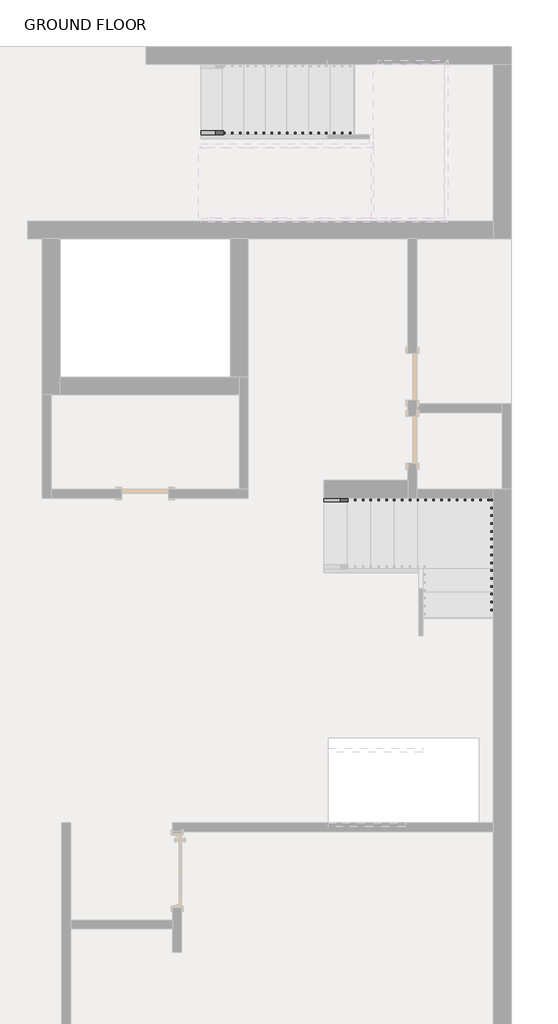
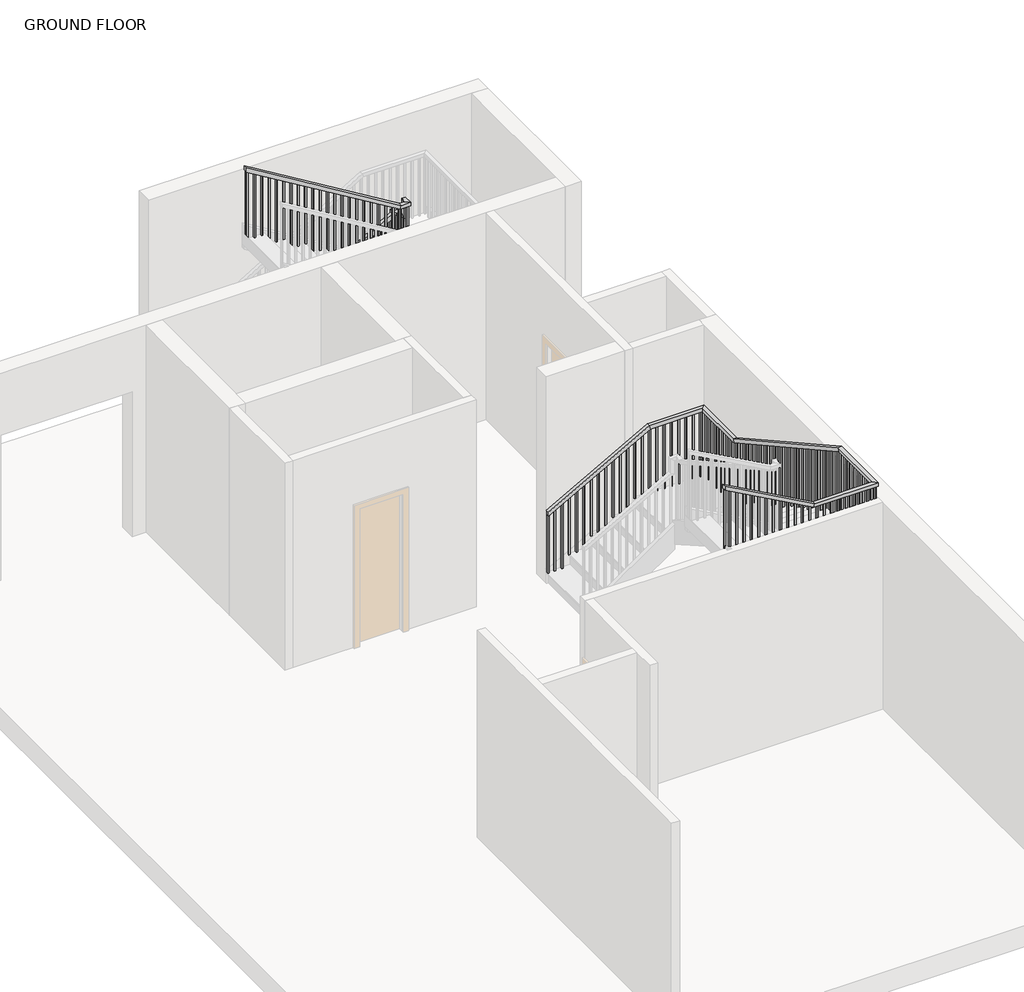
# One storey, part 2 of 3: 2 railings.
"""IFC4 building model written with IfcOpenShell, lengths in millimetres."""

from ifc_helpers import new_model, si_unit, frame, origin, place, context, project, spatial, polyline, outline, extrude, faceted_brep, element, save

model = new_model("IFC4")

# Units and contexts
model_context = context("Model", 3, world=origin())
ifc_project = project(units=[si_unit("LENGTHUNIT", "METRE", prefix="MILLI")], contexts=[model_context])

# Site, building, storey
site = spatial("IfcSite", under=ifc_project)
building = spatial("IfcBuilding", under=site)
storey = spatial("IfcBuildingStorey", under=building, Name="GROUND FLOOR", Elevation=304.8)

# Railings
placement = place(None, origin())
element("IfcRailing", 1, ObjectType="Handrail - Rectangular", at=placement, inside=storey, context=model_context, shape_type="SolidModel", body=[
    faceted_brep([(-12941.4571222, 6804.8964313, 1388.5333333), (-12941.4571222, 6804.8964313, 1329.1318731), (-12941.4571222, 6754.0964313, 1329.1318731), (-12941.4571222, 6754.0964313, 1388.5333333), (-10782.4571222, 6804.8964313, 2697.0181818), (-10731.6571222, 6804.8964313, 2668.4046004), (-10731.6571222, 6754.0964313, 2668.4046004), (-10782.4571222, 6754.0964313, 2697.0181818), (-10782.4571222, 6804.8964313, 2743.2), (-10731.6571222, 6804.8964313, 2692.4), (-10731.6571222, 6754.0964313, 2692.4), (-10782.4571222, 6754.0964313, 2743.2), (-10655.4571222, 6804.8964313, 2743.2), (-10655.4571222, 6804.8964313, 2692.4), (-10706.2571222, 6754.0964313, 2692.4), (-10706.2571222, 6754.0964313, 2743.2), (-10655.4571222, 6677.8964313, 2743.2), (-10655.4571222, 6677.8964313, 2692.4), (-10706.2571222, 6677.8964313, 2692.4), (-10706.2571222, 6677.8964313, 2743.2), (-10655.4571222, 6663.5776214, 2743.2), (-10655.4571222, 6612.7776214, 2692.4), (-10706.2571222, 6612.7776214, 2692.4), (-10706.2571222, 6663.5776214, 2743.2), (-10655.4571222, 6663.5776214, 2958.7151515), (-10655.4571222, 6612.7776214, 2907.9151515), (-10706.2571222, 6612.7776214, 2907.9151515), (-10706.2571222, 6663.5776214, 2958.7151515), (-10655.4571222, 6536.5776214, 2958.7151515), (-10655.4571222, 6536.5776214, 2907.9151515), (-10706.2571222, 6587.3776214, 2907.9151515), (-10706.2571222, 6587.3776214, 2958.7151515), (-10782.4571222, 6536.5776214, 2958.7151515), (-10796.6495316, 6536.5776214, 2907.9151515), (-10796.6495316, 6587.3776214, 2907.9151515), (-10782.4571222, 6587.3776214, 2958.7151515), (-12941.4571222, 6536.5776214, 4267.2), (-12941.4571222, 6587.3776214, 4267.2), (-12941.4571222, 6587.3776214, 4207.7985397), (-12941.4571222, 6536.5776214, 4207.7985397)], [[[0, 1, 2, 3]], [[1, 0, 4, 5]], [[2, 1, 5, 6]], [[3, 2, 6, 7]], [[0, 3, 7, 4]], [[5, 4, 8, 9]], [[6, 5, 9, 10]], [[7, 6, 10, 11]], [[4, 7, 11, 8]], [[9, 8, 12, 13]], [[10, 9, 13, 14]], [[11, 10, 14, 15]], [[8, 11, 15, 12]], [[13, 12, 16, 17]], [[14, 13, 17, 18]], [[15, 14, 18, 19]], [[12, 15, 19, 16]], [[17, 16, 20, 21]], [[18, 17, 21, 22]], [[19, 18, 22, 23]], [[16, 19, 23, 20]], [[21, 20, 24, 25]], [[22, 21, 25, 26]], [[23, 22, 26, 27]], [[20, 23, 27, 24]], [[25, 24, 28, 29]], [[26, 25, 29, 30]], [[27, 26, 30, 31]], [[24, 27, 31, 28]], [[29, 28, 32, 33]], [[30, 29, 33, 34]], [[31, 30, 34, 35]], [[28, 31, 35, 32]], [[36, 37, 38, 39]], [[33, 32, 36, 39]], [[34, 33, 39, 38]], [[35, 34, 38, 37]], [[32, 35, 37, 36]]]),
    extrude(outline(polyline([(4186.6318731, -12906.5321222), (4198.1773276, -12925.5821222), (3183.4666667, -12925.5821222), (3183.4666667, -12906.5321222), (4186.6318731, -12906.5321222)])), frame((0.0, 6552.4526214, 0.0), z_axis=(0.0, 1.0, 0.0), x_axis=(0.0, 0.0, 1.0)), (0.0, 0.0, 1.0), 19.05),
    extrude(outline(polyline([(4125.0561155, -12804.9321222), (4136.60157, -12823.9821222), (3183.4666667, -12823.9821222), (3183.4666667, -12804.9321222), (4125.0561155, -12804.9321222)])), frame((0.0, 6552.4526214, 0.0), z_axis=(0.0, 1.0, 0.0), x_axis=(0.0, 0.0, 1.0)), (0.0, 0.0, 1.0), 19.05),
    extrude(outline(polyline([(4063.4803579, -12703.3321222), (4075.0258125, -12722.3821222), (3183.4666667, -12722.3821222), (3183.4666667, -12703.3321222), (4063.4803579, -12703.3321222)])), frame((0.0, 6552.4526214, 0.0), z_axis=(0.0, 1.0, 0.0), x_axis=(0.0, 0.0, 1.0)), (0.0, 0.0, 1.0), 19.05),
    extrude(outline(polyline([(4001.9046004, -12601.7321222), (4013.4500549, -12620.7821222), (3014.1333333, -12620.7821222), (3014.1333333, -12601.7321222), (4001.9046004, -12601.7321222)])), frame((0.0, 6552.4526214, 0.0), z_axis=(0.0, 1.0, 0.0), x_axis=(0.0, 0.0, 1.0)), (0.0, 0.0, 1.0), 19.05),
    extrude(outline(polyline([(3940.3288428, -12500.1321222), (3951.8742973, -12519.1821222), (3014.1333333, -12519.1821222), (3014.1333333, -12500.1321222), (3940.3288428, -12500.1321222)])), frame((0.0, 6552.4526214, 0.0), z_axis=(0.0, 1.0, 0.0), x_axis=(0.0, 0.0, 1.0)), (0.0, 0.0, 1.0), 19.05),
    extrude(outline(polyline([(3878.7530852, -12398.5321222), (3890.2985397, -12417.5821222), (3014.1333333, -12417.5821222), (3014.1333333, -12398.5321222), (3878.7530852, -12398.5321222)])), frame((0.0, 6552.4526214, 0.0), z_axis=(0.0, 1.0, 0.0), x_axis=(0.0, 0.0, 1.0)), (0.0, 0.0, 1.0), 19.05),
    extrude(outline(polyline([(3817.1773276, -12296.9321222), (3828.7227822, -12315.9821222), (2844.8, -12315.9821222), (2844.8, -12296.9321222), (3817.1773276, -12296.9321222)])), frame((0.0, 6552.4526214, 0.0), z_axis=(0.0, 1.0, 0.0), x_axis=(0.0, 0.0, 1.0)), (0.0, 0.0, 1.0), 19.05),
    extrude(outline(polyline([(3755.60157, -12195.3321222), (3767.1470246, -12214.3821222), (2844.8, -12214.3821222), (2844.8, -12195.3321222), (3755.60157, -12195.3321222)])), frame((0.0, 6552.4526214, 0.0), z_axis=(0.0, 1.0, 0.0), x_axis=(0.0, 0.0, 1.0)), (0.0, 0.0, 1.0), 19.05),
    extrude(outline(polyline([(3694.0258125, -12093.7321222), (3705.571267, -12112.7821222), (2844.8, -12112.7821222), (2844.8, -12093.7321222), (3694.0258125, -12093.7321222)])), frame((0.0, 6552.4526214, 0.0), z_axis=(0.0, 1.0, 0.0), x_axis=(0.0, 0.0, 1.0)), (0.0, 0.0, 1.0), 19.05),
    extrude(outline(polyline([(3632.4500549, -11992.1321222), (3643.9955094, -12011.1821222), (2675.4666667, -12011.1821222), (2675.4666667, -11992.1321222), (3632.4500549, -11992.1321222)])), frame((0.0, 6552.4526214, 0.0), z_axis=(0.0, 1.0, 0.0), x_axis=(0.0, 0.0, 1.0)), (0.0, 0.0, 1.0), 19.05),
    extrude(outline(polyline([(3570.8742973, -11890.5321222), (3582.4197519, -11909.5821222), (2675.4666667, -11909.5821222), (2675.4666667, -11890.5321222), (3570.8742973, -11890.5321222)])), frame((0.0, 6552.4526214, 0.0), z_axis=(0.0, 1.0, 0.0), x_axis=(0.0, 0.0, 1.0)), (0.0, 0.0, 1.0), 19.05),
    extrude(outline(polyline([(3509.2985397, -11788.9321222), (3520.8439943, -11807.9821222), (2506.1333333, -11807.9821222), (2506.1333333, -11788.9321222), (3509.2985397, -11788.9321222)])), frame((0.0, 6552.4526214, 0.0), z_axis=(0.0, 1.0, 0.0), x_axis=(0.0, 0.0, 1.0)), (0.0, 0.0, 1.0), 19.05),
    extrude(outline(polyline([(3447.7227822, -11687.3321222), (3459.2682367, -11706.3821222), (2506.1333333, -11706.3821222), (2506.1333333, -11687.3321222), (3447.7227822, -11687.3321222)])), frame((0.0, 6552.4526214, 0.0), z_axis=(0.0, 1.0, 0.0), x_axis=(0.0, 0.0, 1.0)), (0.0, 0.0, 1.0), 19.05),
    extrude(outline(polyline([(3386.1470246, -11585.7321222), (3397.6924791, -11604.7821222), (2506.1333333, -11604.7821222), (2506.1333333, -11585.7321222), (3386.1470246, -11585.7321222)])), frame((0.0, 6552.4526214, 0.0), z_axis=(0.0, 1.0, 0.0), x_axis=(0.0, 0.0, 1.0)), (0.0, 0.0, 1.0), 19.05),
    extrude(outline(polyline([(3324.571267, -11484.1321222), (3336.1167216, -11503.1821222), (2336.8, -11503.1821222), (2336.8, -11484.1321222), (3324.571267, -11484.1321222)])), frame((0.0, 6552.4526214, 0.0), z_axis=(0.0, 1.0, 0.0), x_axis=(0.0, 0.0, 1.0)), (0.0, 0.0, 1.0), 19.05),
    extrude(outline(polyline([(3262.9955094, -11382.5321222), (3274.540964, -11401.5821222), (2336.8, -11401.5821222), (2336.8, -11382.5321222), (3262.9955094, -11382.5321222)])), frame((0.0, 6552.4526214, 0.0), z_axis=(0.0, 1.0, 0.0), x_axis=(0.0, 0.0, 1.0)), (0.0, 0.0, 1.0), 19.05),
    extrude(outline(polyline([(3201.4197519, -11280.9321222), (3212.9652064, -11299.9821222), (2336.8, -11299.9821222), (2336.8, -11280.9321222), (3201.4197519, -11280.9321222)])), frame((0.0, 6552.4526214, 0.0), z_axis=(0.0, 1.0, 0.0), x_axis=(0.0, 0.0, 1.0)), (0.0, 0.0, 1.0), 19.05),
    extrude(outline(polyline([(3139.8439943, -11179.3321222), (3151.3894488, -11198.3821222), (2167.4666667, -11198.3821222), (2167.4666667, -11179.3321222), (3139.8439943, -11179.3321222)])), frame((0.0, 6552.4526214, 0.0), z_axis=(0.0, 1.0, 0.0), x_axis=(0.0, 0.0, 1.0)), (0.0, 0.0, 1.0), 19.05),
    extrude(outline(polyline([(3078.2682367, -11077.7321222), (3089.8136913, -11096.7821222), (2167.4666667, -11096.7821222), (2167.4666667, -11077.7321222), (3078.2682367, -11077.7321222)])), frame((0.0, 6552.4526214, 0.0), z_axis=(0.0, 1.0, 0.0), x_axis=(0.0, 0.0, 1.0)), (0.0, 0.0, 1.0), 19.05),
    extrude(outline(polyline([(3016.6924791, -10976.1321222), (3028.2379337, -10995.1821222), (2167.4666667, -10995.1821222), (2167.4666667, -10976.1321222), (3016.6924791, -10976.1321222)])), frame((0.0, 6552.4526214, 0.0), z_axis=(0.0, 1.0, 0.0), x_axis=(0.0, 0.0, 1.0)), (0.0, 0.0, 1.0), 19.05),
    extrude(outline(polyline([(2955.1167216, -10874.5321222), (2966.6621761, -10893.5821222), (1998.1333333, -10893.5821222), (1998.1333333, -10874.5321222), (2955.1167216, -10874.5321222)])), frame((0.0, 6552.4526214, 0.0), z_axis=(0.0, 1.0, 0.0), x_axis=(0.0, 0.0, 1.0)), (0.0, 0.0, 1.0), 19.05),
    extrude(outline(polyline([(2893.540964, -10772.9321222), (2905.0864185, -10791.9821222), (1998.1333333, -10791.9821222), (1998.1333333, -10772.9321222), (2893.540964, -10772.9321222)])), frame((0.0, 6552.4526214, 0.0), z_axis=(0.0, 1.0, 0.0), x_axis=(0.0, 0.0, 1.0)), (0.0, 0.0, 1.0), 19.05),
    extrude(outline(polyline([(-10690.3821222, 6585.8214313), (-10671.3321222, 6585.8214313), (-10671.3321222, 6566.7714313), (-10690.3821222, 6566.7714313), (-10690.3821222, 6585.8214313)])), frame((0.0, 0.0, 1828.8), z_axis=(0.0, 0.0, 1.0), x_axis=(1.0, 0.0, 0.0)), (0.0, 0.0, 1.0), 1079.1151515),
    extrude(outline(polyline([(-10690.3821222, 6687.4214313), (-10671.3321222, 6687.4214313), (-10671.3321222, 6668.3714313), (-10690.3821222, 6668.3714313), (-10690.3821222, 6687.4214313)])), frame((0.0, 0.0, 1828.8), z_axis=(0.0, 0.0, 1.0), x_axis=(1.0, 0.0, 0.0)), (0.0, 0.0, 1.0), 863.6),
    extrude(outline(polyline([(-10715.7821222, 6769.9714313), (-10715.7821222, 6789.0214313), (-10696.7321222, 6789.0214313), (-10696.7321222, 6769.9714313), (-10715.7821222, 6769.9714313)])), frame((0.0, 0.0, 1828.8), z_axis=(0.0, 0.0, 1.0), x_axis=(1.0, 0.0, 0.0)), (0.0, 0.0, 1.0), 863.6),
    extrude(outline(polyline([(2627.9955094, -10798.3321222), (2616.4500549, -10817.3821222), (1659.4666667, -10817.3821222), (1659.4666667, -10798.3321222), (2627.9955094, -10798.3321222)])), frame((0.0, 6769.9714313, 0.0), z_axis=(0.0, 1.0, 0.0), x_axis=(0.0, 0.0, 1.0)), (0.0, 0.0, 1.0), 19.05),
    extrude(outline(polyline([(2566.4197519, -10899.9321222), (2554.8742973, -10918.9821222), (1659.4666667, -10918.9821222), (1659.4666667, -10899.9321222), (2566.4197519, -10899.9321222)])), frame((0.0, 6769.9714313, 0.0), z_axis=(0.0, 1.0, 0.0), x_axis=(0.0, 0.0, 1.0)), (0.0, 0.0, 1.0), 19.05),
    extrude(outline(polyline([(2504.8439943, -11001.5321222), (2493.2985397, -11020.5821222), (1490.1333333, -11020.5821222), (1490.1333333, -11001.5321222), (2504.8439943, -11001.5321222)])), frame((0.0, 6769.9714313, 0.0), z_axis=(0.0, 1.0, 0.0), x_axis=(0.0, 0.0, 1.0)), (0.0, 0.0, 1.0), 19.05),
    extrude(outline(polyline([(2443.2682367, -11103.1321222), (2431.7227822, -11122.1821222), (1490.1333333, -11122.1821222), (1490.1333333, -11103.1321222), (2443.2682367, -11103.1321222)])), frame((0.0, 6769.9714313, 0.0), z_axis=(0.0, 1.0, 0.0), x_axis=(0.0, 0.0, 1.0)), (0.0, 0.0, 1.0), 19.05),
    extrude(outline(polyline([(2381.6924791, -11204.7321222), (2370.1470246, -11223.7821222), (1490.1333333, -11223.7821222), (1490.1333333, -11204.7321222), (2381.6924791, -11204.7321222)])), frame((0.0, 6769.9714313, 0.0), z_axis=(0.0, 1.0, 0.0), x_axis=(0.0, 0.0, 1.0)), (0.0, 0.0, 1.0), 19.05),
    extrude(outline(polyline([(2320.1167216, -11306.3321222), (2308.571267, -11325.3821222), (1320.8, -11325.3821222), (1320.8, -11306.3321222), (2320.1167216, -11306.3321222)])), frame((0.0, 6769.9714313, 0.0), z_axis=(0.0, 1.0, 0.0), x_axis=(0.0, 0.0, 1.0)), (0.0, 0.0, 1.0), 19.05),
    extrude(outline(polyline([(2258.540964, -11407.9321222), (2246.9955094, -11426.9821222), (1320.8, -11426.9821222), (1320.8, -11407.9321222), (2258.540964, -11407.9321222)])), frame((0.0, 6769.9714313, 0.0), z_axis=(0.0, 1.0, 0.0), x_axis=(0.0, 0.0, 1.0)), (0.0, 0.0, 1.0), 19.05),
    extrude(outline(polyline([(2196.9652064, -11509.5321222), (2185.4197519, -11528.5821222), (1320.8, -11528.5821222), (1320.8, -11509.5321222), (2196.9652064, -11509.5321222)])), frame((0.0, 6769.9714313, 0.0), z_axis=(0.0, 1.0, 0.0), x_axis=(0.0, 0.0, 1.0)), (0.0, 0.0, 1.0), 19.05),
    extrude(outline(polyline([(2135.3894488, -11611.1321222), (2123.8439943, -11630.1821222), (1151.4666667, -11630.1821222), (1151.4666667, -11611.1321222), (2135.3894488, -11611.1321222)])), frame((0.0, 6769.9714313, 0.0), z_axis=(0.0, 1.0, 0.0), x_axis=(0.0, 0.0, 1.0)), (0.0, 0.0, 1.0), 19.05),
    extrude(outline(polyline([(2073.8136913, -11712.7321222), (2062.2682367, -11731.7821222), (1151.4666667, -11731.7821222), (1151.4666667, -11712.7321222), (2073.8136913, -11712.7321222)])), frame((0.0, 6769.9714313, 0.0), z_axis=(0.0, 1.0, 0.0), x_axis=(0.0, 0.0, 1.0)), (0.0, 0.0, 1.0), 19.05),
    extrude(outline(polyline([(2012.2379337, -11814.3321222), (2000.6924791, -11833.3821222), (1151.4666667, -11833.3821222), (1151.4666667, -11814.3321222), (2012.2379337, -11814.3321222)])), frame((0.0, 6769.9714313, 0.0), z_axis=(0.0, 1.0, 0.0), x_axis=(0.0, 0.0, 1.0)), (0.0, 0.0, 1.0), 19.05),
    extrude(outline(polyline([(1950.6621761, -11915.9321222), (1939.1167216, -11934.9821222), (982.1333333, -11934.9821222), (982.1333333, -11915.9321222), (1950.6621761, -11915.9321222)])), frame((0.0, 6769.9714313, 0.0), z_axis=(0.0, 1.0, 0.0), x_axis=(0.0, 0.0, 1.0)), (0.0, 0.0, 1.0), 19.05),
    extrude(outline(polyline([(1889.0864185, -12017.5321222), (1877.540964, -12036.5821222), (982.1333333, -12036.5821222), (982.1333333, -12017.5321222), (1889.0864185, -12017.5321222)])), frame((0.0, 6769.9714313, 0.0), z_axis=(0.0, 1.0, 0.0), x_axis=(0.0, 0.0, 1.0)), (0.0, 0.0, 1.0), 19.05),
    extrude(outline(polyline([(1827.510661, -12119.1321222), (1815.9652064, -12138.1821222), (812.8, -12138.1821222), (812.8, -12119.1321222), (1827.510661, -12119.1321222)])), frame((0.0, 6769.9714313, 0.0), z_axis=(0.0, 1.0, 0.0), x_axis=(0.0, 0.0, 1.0)), (0.0, 0.0, 1.0), 19.05),
    extrude(outline(polyline([(1765.9349034, -12220.7321222), (1754.3894488, -12239.7821222), (812.8, -12239.7821222), (812.8, -12220.7321222), (1765.9349034, -12220.7321222)])), frame((0.0, 6769.9714313, 0.0), z_axis=(0.0, 1.0, 0.0), x_axis=(0.0, 0.0, 1.0)), (0.0, 0.0, 1.0), 19.05),
    extrude(outline(polyline([(1704.3591458, -12322.3321222), (1692.8136913, -12341.3821222), (812.8, -12341.3821222), (812.8, -12322.3321222), (1704.3591458, -12322.3321222)])), frame((0.0, 6769.9714313, 0.0), z_axis=(0.0, 1.0, 0.0), x_axis=(0.0, 0.0, 1.0)), (0.0, 0.0, 1.0), 19.05),
    extrude(outline(polyline([(1642.7833882, -12423.9321222), (1631.2379337, -12442.9821222), (643.4666667, -12442.9821222), (643.4666667, -12423.9321222), (1642.7833882, -12423.9321222)])), frame((0.0, 6769.9714313, 0.0), z_axis=(0.0, 1.0, 0.0), x_axis=(0.0, 0.0, 1.0)), (0.0, 0.0, 1.0), 19.05),
    extrude(outline(polyline([(1581.2076307, -12525.5321222), (1569.6621761, -12544.5821222), (643.4666667, -12544.5821222), (643.4666667, -12525.5321222), (1581.2076307, -12525.5321222)])), frame((0.0, 6769.9714313, 0.0), z_axis=(0.0, 1.0, 0.0), x_axis=(0.0, 0.0, 1.0)), (0.0, 0.0, 1.0), 19.05),
    extrude(outline(polyline([(1519.6318731, -12627.1321222), (1508.0864185, -12646.1821222), (643.4666667, -12646.1821222), (643.4666667, -12627.1321222), (1519.6318731, -12627.1321222)])), frame((0.0, 6769.9714313, 0.0), z_axis=(0.0, 1.0, 0.0), x_axis=(0.0, 0.0, 1.0)), (0.0, 0.0, 1.0), 19.05),
    extrude(outline(polyline([(1458.0561155, -12728.7321222), (1446.510661, -12747.7821222), (474.1333333, -12747.7821222), (474.1333333, -12728.7321222), (1458.0561155, -12728.7321222)])), frame((0.0, 6769.9714313, 0.0), z_axis=(0.0, 1.0, 0.0), x_axis=(0.0, 0.0, 1.0)), (0.0, 0.0, 1.0), 19.05),
    extrude(outline(polyline([(1396.4803579, -12830.3321222), (1384.9349034, -12849.3821222), (474.1333333, -12849.3821222), (474.1333333, -12830.3321222), (1396.4803579, -12830.3321222)])), frame((0.0, 6769.9714313, 0.0), z_axis=(0.0, 1.0, 0.0), x_axis=(0.0, 0.0, 1.0)), (0.0, 0.0, 1.0), 19.05),
    extrude(outline(polyline([(-10690.3821222, 6571.5026214), (-10671.3321222, 6571.5026214), (-10671.3321222, 6552.4526214), (-10690.3821222, 6552.4526214), (-10690.3821222, 6571.5026214)])), frame((0.0, 0.0, 1828.8), z_axis=(0.0, 0.0, 1.0), x_axis=(1.0, 0.0, 0.0)), (0.0, 0.0, 1.0), 1079.1151515),
    extrude(outline(polyline([(-10690.3821222, 6769.9714313), (-10690.3821222, 6789.0214313), (-10671.3321222, 6789.0214313), (-10671.3321222, 6769.9714313), (-10690.3821222, 6769.9714313)])), frame((0.0, 0.0, 1828.8), z_axis=(0.0, 0.0, 1.0), x_axis=(1.0, 0.0, 0.0)), (0.0, 0.0, 1.0), 863.6),
    extrude(outline(polyline([(4196.2530852, -12922.4071222), (4207.7985397, -12941.4571222), (3183.4666667, -12941.4571222), (3183.4666667, -12922.4071222), (4196.2530852, -12922.4071222)])), frame((0.0, 6552.4526214, 0.0), z_axis=(0.0, 1.0, 0.0), x_axis=(0.0, 0.0, 1.0)), (0.0, 0.0, 1.0), 19.05),
    extrude(outline(polyline([(1340.6773276, -12922.4071222), (1329.1318731, -12941.4571222), (474.1333333, -12941.4571222), (474.1333333, -12922.4071222), (1340.6773276, -12922.4071222)])), frame((0.0, 6769.9714313, 0.0), z_axis=(0.0, 1.0, 0.0), x_axis=(0.0, 0.0, 1.0)), (0.0, 0.0, 1.0), 19.05),
])
element("IfcRailing", 2, ObjectType="Handrail - Rectangular", at=placement, inside=storey, context=model_context, shape_type="SolidModel", body=[
    faceted_brep([(-11350.6229553, 2055.0964313, 1388.5333333), (-11350.6229553, 2055.0964313, 1330.420221), (-11350.6229553, 2004.2964313, 1330.420221), (-11350.6229553, 2004.2964313, 1388.5333333), (-9947.2729553, 2055.0964313, 2168.1722222), (-9934.109353, 2055.0964313, 2117.3722222), (-9934.109353, 2004.2964313, 2117.3722222), (-9947.2729553, 2004.2964313, 2168.1722222), (-9153.5229553, 2055.0964313, 2168.1722222), (-9153.5229553, 2055.0964313, 2117.3722222), (-9204.3229553, 2004.2964313, 2117.3722222), (-9204.3229553, 2004.2964313, 2168.1722222), (-9153.5229553, 1261.3464313, 2168.1722222), (-9153.5229553, 1248.1828291, 2117.3722222), (-9204.3229553, 1248.1828291, 2117.3722222), (-9204.3229553, 1261.3464313, 2168.1722222), (-9153.5229553, -1265.9535687, 3572.2277778), (-9153.5229553, -1279.1171709, 3521.4277778), (-9204.3229553, -1279.1171709, 3521.4277778), (-9204.3229553, -1265.9535687, 3572.2277778), (-9153.5229553, -2148.6035687, 3572.2277778), (-9153.5229553, -2148.6035687, 3521.4277778), (-9204.3229553, -2097.8035687, 3521.4277778), (-9204.3229553, -2097.8035687, 3572.2277778), (-10036.1729553, -2148.6035687, 3572.2277778), (-10049.3365575, -2148.6035687, 3521.4277778), (-10049.3365575, -2097.8035687, 3521.4277778), (-10036.1729553, -2097.8035687, 3572.2277778), (-11287.1229553, -2148.6035687, 4267.2), (-11287.1229553, -2097.8035687, 4267.2), (-11287.1229553, -2097.8035687, 4209.0868876), (-11287.1229553, -2148.6035687, 4209.0868876)], [[[0, 1, 2, 3]], [[1, 0, 4, 5]], [[2, 1, 5, 6]], [[3, 2, 6, 7]], [[0, 3, 7, 4]], [[5, 4, 8, 9]], [[6, 5, 9, 10]], [[7, 6, 10, 11]], [[4, 7, 11, 8]], [[9, 8, 12, 13]], [[10, 9, 13, 14]], [[11, 10, 14, 15]], [[8, 11, 15, 12]], [[13, 12, 16, 17]], [[14, 13, 17, 18]], [[15, 14, 18, 19]], [[12, 15, 19, 16]], [[17, 16, 20, 21]], [[18, 17, 21, 22]], [[19, 18, 22, 23]], [[16, 19, 23, 20]], [[21, 20, 24, 25]], [[22, 21, 25, 26]], [[23, 22, 26, 27]], [[20, 23, 27, 24]], [[28, 29, 30, 31]], [[25, 24, 28, 31]], [[26, 25, 31, 30]], [[27, 26, 30, 29]], [[24, 27, 29, 28]]]),
    extrude(outline(polyline([(4172.045221, -11220.4479553), (3183.4666667, -11220.4479553), (3183.4666667, -11201.3979553), (4161.4618876, -11201.3979553), (4172.045221, -11220.4479553)])), frame((0.0, -2132.7285687, 0.0), z_axis=(0.0, 1.0, 0.0), x_axis=(0.0, 0.0, 1.0)), (0.0, 0.0, 1.0), 19.05),
    extrude(outline(polyline([(4115.6007765, -11118.8479553), (3183.4666667, -11118.8479553), (3183.4666667, -11099.7979553), (4105.0174432, -11099.7979553), (4115.6007765, -11118.8479553)])), frame((0.0, -2132.7285687, 0.0), z_axis=(0.0, 1.0, 0.0), x_axis=(0.0, 0.0, 1.0)), (0.0, 0.0, 1.0), 19.05),
    extrude(outline(polyline([(4059.1563321, -11017.2479553), (3183.4666667, -11017.2479553), (3183.4666667, -10998.1979553), (4048.5729988, -10998.1979553), (4059.1563321, -11017.2479553)])), frame((0.0, -2132.7285687, 0.0), z_axis=(0.0, 1.0, 0.0), x_axis=(0.0, 0.0, 1.0)), (0.0, 0.0, 1.0), 19.05),
    extrude(outline(polyline([(4002.7118876, -10915.6479553), (3014.1333333, -10915.6479553), (3014.1333333, -10896.5979553), (3992.1285543, -10896.5979553), (4002.7118876, -10915.6479553)])), frame((0.0, -2132.7285687, 0.0), z_axis=(0.0, 1.0, 0.0), x_axis=(0.0, 0.0, 1.0)), (0.0, 0.0, 1.0), 19.05),
    extrude(outline(polyline([(3946.2674432, -10814.0479553), (3014.1333333, -10814.0479553), (3014.1333333, -10794.9979553), (3935.6841099, -10794.9979553), (3946.2674432, -10814.0479553)])), frame((0.0, -2132.7285687, 0.0), z_axis=(0.0, 1.0, 0.0), x_axis=(0.0, 0.0, 1.0)), (0.0, 0.0, 1.0), 19.05),
    extrude(outline(polyline([(3889.8229988, -10712.4479553), (3014.1333333, -10712.4479553), (3014.1333333, -10693.3979553), (3879.2396654, -10693.3979553), (3889.8229988, -10712.4479553)])), frame((0.0, -2132.7285687, 0.0), z_axis=(0.0, 1.0, 0.0), x_axis=(0.0, 0.0, 1.0)), (0.0, 0.0, 1.0), 19.05),
    extrude(outline(polyline([(3833.3785543, -10610.8479553), (2844.8, -10610.8479553), (2844.8, -10591.7979553), (3822.795221, -10591.7979553), (3833.3785543, -10610.8479553)])), frame((0.0, -2132.7285687, 0.0), z_axis=(0.0, 1.0, 0.0), x_axis=(0.0, 0.0, 1.0)), (0.0, 0.0, 1.0), 19.05),
    extrude(outline(polyline([(3776.9341099, -10509.2479553), (2844.8, -10509.2479553), (2844.8, -10490.1979553), (3766.3507765, -10490.1979553), (3776.9341099, -10509.2479553)])), frame((0.0, -2132.7285687, 0.0), z_axis=(0.0, 1.0, 0.0), x_axis=(0.0, 0.0, 1.0)), (0.0, 0.0, 1.0), 19.05),
    extrude(outline(polyline([(3720.4896654, -10407.6479553), (2844.8, -10407.6479553), (2844.8, -10388.5979553), (3709.9063321, -10388.5979553), (3720.4896654, -10407.6479553)])), frame((0.0, -2132.7285687, 0.0), z_axis=(0.0, 1.0, 0.0), x_axis=(0.0, 0.0, 1.0)), (0.0, 0.0, 1.0), 19.05),
    extrude(outline(polyline([(3664.045221, -10306.0479553), (2675.4666667, -10306.0479553), (2675.4666667, -10286.9979553), (3653.4618876, -10286.9979553), (3664.045221, -10306.0479553)])), frame((0.0, -2132.7285687, 0.0), z_axis=(0.0, 1.0, 0.0), x_axis=(0.0, 0.0, 1.0)), (0.0, 0.0, 1.0), 19.05),
    extrude(outline(polyline([(3607.6007765, -10204.4479553), (2675.4666667, -10204.4479553), (2675.4666667, -10185.3979553), (3597.0174432, -10185.3979553), (3607.6007765, -10204.4479553)])), frame((0.0, -2132.7285687, 0.0), z_axis=(0.0, 1.0, 0.0), x_axis=(0.0, 0.0, 1.0)), (0.0, 0.0, 1.0), 19.05),
    extrude(outline(polyline([(3551.1563321, -10102.8479553), (2675.4666667, -10102.8479553), (2675.4666667, -10083.7979553), (3540.5729988, -10083.7979553), (3551.1563321, -10102.8479553)])), frame((0.0, -2132.7285687, 0.0), z_axis=(0.0, 1.0, 0.0), x_axis=(0.0, 0.0, 1.0)), (0.0, 0.0, 1.0), 19.05),
    extrude(outline(polyline([(-9982.1979553, -2132.7285687), (-10001.2479553, -2132.7285687), (-10001.2479553, -2113.6785687), (-9982.1979553, -2113.6785687), (-9982.1979553, -2132.7285687)])), frame((0.0, 0.0, 2506.1333333), z_axis=(0.0, 0.0, 1.0), x_axis=(1.0, 0.0, 0.0)), (0.0, 0.0, 1.0), 1015.2944444),
    extrude(outline(polyline([(-9880.5979553, -2132.7285687), (-9899.6479553, -2132.7285687), (-9899.6479553, -2113.6785687), (-9880.5979553, -2113.6785687), (-9880.5979553, -2132.7285687)])), frame((0.0, 0.0, 2506.1333333), z_axis=(0.0, 0.0, 1.0), x_axis=(1.0, 0.0, 0.0)), (0.0, 0.0, 1.0), 1015.2944444),
    extrude(outline(polyline([(-9778.9979553, -2132.7285687), (-9798.0479553, -2132.7285687), (-9798.0479553, -2113.6785687), (-9778.9979553, -2113.6785687), (-9778.9979553, -2132.7285687)])), frame((0.0, 0.0, 2506.1333333), z_axis=(0.0, 0.0, 1.0), x_axis=(1.0, 0.0, 0.0)), (0.0, 0.0, 1.0), 1015.2944444),
    extrude(outline(polyline([(-9677.3979553, -2132.7285687), (-9696.4479553, -2132.7285687), (-9696.4479553, -2113.6785687), (-9677.3979553, -2113.6785687), (-9677.3979553, -2132.7285687)])), frame((0.0, 0.0, 2506.1333333), z_axis=(0.0, 0.0, 1.0), x_axis=(1.0, 0.0, 0.0)), (0.0, 0.0, 1.0), 1015.2944444),
    extrude(outline(polyline([(-9575.7979553, -2132.7285687), (-9594.8479553, -2132.7285687), (-9594.8479553, -2113.6785687), (-9575.7979553, -2113.6785687), (-9575.7979553, -2132.7285687)])), frame((0.0, 0.0, 2506.1333333), z_axis=(0.0, 0.0, 1.0), x_axis=(1.0, 0.0, 0.0)), (0.0, 0.0, 1.0), 1015.2944444),
    extrude(outline(polyline([(-9474.1979553, -2132.7285687), (-9493.2479553, -2132.7285687), (-9493.2479553, -2113.6785687), (-9474.1979553, -2113.6785687), (-9474.1979553, -2132.7285687)])), frame((0.0, 0.0, 2506.1333333), z_axis=(0.0, 0.0, 1.0), x_axis=(1.0, 0.0, 0.0)), (0.0, 0.0, 1.0), 1015.2944444),
    extrude(outline(polyline([(-9372.5979553, -2132.7285687), (-9391.6479553, -2132.7285687), (-9391.6479553, -2113.6785687), (-9372.5979553, -2113.6785687), (-9372.5979553, -2132.7285687)])), frame((0.0, 0.0, 2506.1333333), z_axis=(0.0, 0.0, 1.0), x_axis=(1.0, 0.0, 0.0)), (0.0, 0.0, 1.0), 1015.2944444),
    extrude(outline(polyline([(-9270.9979553, -2132.7285687), (-9290.0479553, -2132.7285687), (-9290.0479553, -2113.6785687), (-9270.9979553, -2113.6785687), (-9270.9979553, -2132.7285687)])), frame((0.0, 0.0, 2506.1333333), z_axis=(0.0, 0.0, 1.0), x_axis=(1.0, 0.0, 0.0)), (0.0, 0.0, 1.0), 1015.2944444),
    extrude(outline(polyline([(-9169.3979553, -2024.7785687), (-9169.3979553, -2043.8285687), (-9188.4479553, -2043.8285687), (-9188.4479553, -2024.7785687), (-9169.3979553, -2024.7785687)])), frame((0.0, 0.0, 2506.1333333), z_axis=(0.0, 0.0, 1.0), x_axis=(1.0, 0.0, 0.0)), (0.0, 0.0, 1.0), 1015.2944444),
    extrude(outline(polyline([(-9169.3979553, -1923.1785687), (-9169.3979553, -1942.2285687), (-9188.4479553, -1942.2285687), (-9188.4479553, -1923.1785687), (-9169.3979553, -1923.1785687)])), frame((0.0, 0.0, 2506.1333333), z_axis=(0.0, 0.0, 1.0), x_axis=(1.0, 0.0, 0.0)), (0.0, 0.0, 1.0), 1015.2944444),
    extrude(outline(polyline([(-9169.3979553, -1821.5785687), (-9169.3979553, -1840.6285687), (-9188.4479553, -1840.6285687), (-9188.4479553, -1821.5785687), (-9169.3979553, -1821.5785687)])), frame((0.0, 0.0, 2506.1333333), z_axis=(0.0, 0.0, 1.0), x_axis=(1.0, 0.0, 0.0)), (0.0, 0.0, 1.0), 1015.2944444),
    extrude(outline(polyline([(-9169.3979553, -1719.9785687), (-9169.3979553, -1739.0285687), (-9188.4479553, -1739.0285687), (-9188.4479553, -1719.9785687), (-9169.3979553, -1719.9785687)])), frame((0.0, 0.0, 2506.1333333), z_axis=(0.0, 0.0, 1.0), x_axis=(1.0, 0.0, 0.0)), (0.0, 0.0, 1.0), 1015.2944444),
    extrude(outline(polyline([(-9169.3979553, -1618.3785687), (-9169.3979553, -1637.4285687), (-9188.4479553, -1637.4285687), (-9188.4479553, -1618.3785687), (-9169.3979553, -1618.3785687)])), frame((0.0, 0.0, 2506.1333333), z_axis=(0.0, 0.0, 1.0), x_axis=(1.0, 0.0, 0.0)), (0.0, 0.0, 1.0), 1015.2944444),
    extrude(outline(polyline([(-9169.3979553, -1516.7785687), (-9169.3979553, -1535.8285687), (-9188.4479553, -1535.8285687), (-9188.4479553, -1516.7785687), (-9169.3979553, -1516.7785687)])), frame((0.0, 0.0, 2506.1333333), z_axis=(0.0, 0.0, 1.0), x_axis=(1.0, 0.0, 0.0)), (0.0, 0.0, 1.0), 1015.2944444),
    extrude(outline(polyline([(-9169.3979553, -1415.1785687), (-9169.3979553, -1434.2285687), (-9188.4479553, -1434.2285687), (-9188.4479553, -1415.1785687), (-9169.3979553, -1415.1785687)])), frame((0.0, 0.0, 2506.1333333), z_axis=(0.0, 0.0, 1.0), x_axis=(1.0, 0.0, 0.0)), (0.0, 0.0, 1.0), 1015.2944444),
    extrude(outline(polyline([(-9169.3979553, -1313.5785687), (-9169.3979553, -1332.6285687), (-9188.4479553, -1332.6285687), (-9188.4479553, -1313.5785687), (-9169.3979553, -1313.5785687)])), frame((0.0, 0.0, 2506.1333333), z_axis=(0.0, 0.0, 1.0), x_axis=(1.0, 0.0, 0.0)), (0.0, 0.0, 1.0), 1015.2944444),
    extrude(outline(polyline([(-1211.9785687, 3484.1285543), (-1211.9785687, 2506.1333333), (-1231.0285687, 2506.1333333), (-1231.0285687, 3494.7118876), (-1211.9785687, 3484.1285543)])), frame((-9188.4479553, 0.0, 0.0), z_axis=(1.0, 0.0, 0.0), x_axis=(0.0, 1.0, 0.0)), (0.0, 0.0, 1.0), 19.05),
    extrude(outline(polyline([(-1110.3785687, 3427.6841099), (-1110.3785687, 2506.1333333), (-1129.4285687, 2506.1333333), (-1129.4285687, 3438.2674432), (-1110.3785687, 3427.6841099)])), frame((-9188.4479553, 0.0, 0.0), z_axis=(1.0, 0.0, 0.0), x_axis=(0.0, 1.0, 0.0)), (0.0, 0.0, 1.0), 19.05),
    extrude(outline(polyline([(-1008.7785687, 3371.2396654), (-1008.7785687, 2506.1333333), (-1027.8285687, 2506.1333333), (-1027.8285687, 3381.8229988), (-1008.7785687, 3371.2396654)])), frame((-9188.4479553, 0.0, 0.0), z_axis=(1.0, 0.0, 0.0), x_axis=(0.0, 1.0, 0.0)), (0.0, 0.0, 1.0), 19.05),
    extrude(outline(polyline([(-907.1785687, 3314.795221), (-907.1785687, 2336.8), (-926.2285687, 2336.8), (-926.2285687, 3325.3785543), (-907.1785687, 3314.795221)])), frame((-9188.4479553, 0.0, 0.0), z_axis=(1.0, 0.0, 0.0), x_axis=(0.0, 1.0, 0.0)), (0.0, 0.0, 1.0), 19.05),
    extrude(outline(polyline([(-805.5785687, 3258.3507765), (-805.5785687, 2336.8), (-824.6285687, 2336.8), (-824.6285687, 3268.9341099), (-805.5785687, 3258.3507765)])), frame((-9188.4479553, 0.0, 0.0), z_axis=(1.0, 0.0, 0.0), x_axis=(0.0, 1.0, 0.0)), (0.0, 0.0, 1.0), 19.05),
    extrude(outline(polyline([(-703.9785687, 3201.9063321), (-703.9785687, 2336.8), (-723.0285687, 2336.8), (-723.0285687, 3212.4896654), (-703.9785687, 3201.9063321)])), frame((-9188.4479553, 0.0, 0.0), z_axis=(1.0, 0.0, 0.0), x_axis=(0.0, 1.0, 0.0)), (0.0, 0.0, 1.0), 19.05),
    extrude(outline(polyline([(-602.3785687, 3145.4618876), (-602.3785687, 2167.4666667), (-621.4285687, 2167.4666667), (-621.4285687, 3156.045221), (-602.3785687, 3145.4618876)])), frame((-9188.4479553, 0.0, 0.0), z_axis=(1.0, 0.0, 0.0), x_axis=(0.0, 1.0, 0.0)), (0.0, 0.0, 1.0), 19.05),
    extrude(outline(polyline([(-500.7785687, 3089.0174432), (-500.7785687, 2167.4666667), (-519.8285687, 2167.4666667), (-519.8285687, 3099.6007765), (-500.7785687, 3089.0174432)])), frame((-9188.4479553, 0.0, 0.0), z_axis=(1.0, 0.0, 0.0), x_axis=(0.0, 1.0, 0.0)), (0.0, 0.0, 1.0), 19.05),
    extrude(outline(polyline([(-399.1785687, 3032.5729988), (-399.1785687, 2167.4666667), (-418.2285687, 2167.4666667), (-418.2285687, 3043.1563321), (-399.1785687, 3032.5729988)])), frame((-9188.4479553, 0.0, 0.0), z_axis=(1.0, 0.0, 0.0), x_axis=(0.0, 1.0, 0.0)), (0.0, 0.0, 1.0), 19.05),
    extrude(outline(polyline([(-297.5785687, 2976.1285543), (-297.5785687, 1998.1333333), (-316.6285687, 1998.1333333), (-316.6285687, 2986.7118876), (-297.5785687, 2976.1285543)])), frame((-9188.4479553, 0.0, 0.0), z_axis=(1.0, 0.0, 0.0), x_axis=(0.0, 1.0, 0.0)), (0.0, 0.0, 1.0), 19.05),
    extrude(outline(polyline([(-195.9785687, 2919.6841099), (-195.9785687, 1998.1333333), (-215.0285687, 1998.1333333), (-215.0285687, 2930.2674432), (-195.9785687, 2919.6841099)])), frame((-9188.4479553, 0.0, 0.0), z_axis=(1.0, 0.0, 0.0), x_axis=(0.0, 1.0, 0.0)), (0.0, 0.0, 1.0), 19.05),
    extrude(outline(polyline([(-94.3785687, 2863.2396654), (-94.3785687, 1998.1333333), (-113.4285687, 1998.1333333), (-113.4285687, 2873.8229988), (-94.3785687, 2863.2396654)])), frame((-9188.4479553, 0.0, 0.0), z_axis=(1.0, 0.0, 0.0), x_axis=(0.0, 1.0, 0.0)), (0.0, 0.0, 1.0), 19.05),
    extrude(outline(polyline([(7.2214313, 2806.795221), (7.2214313, 1828.8), (-11.8285687, 1828.8), (-11.8285687, 2817.3785543), (7.2214313, 2806.795221)])), frame((-9188.4479553, 0.0, 0.0), z_axis=(1.0, 0.0, 0.0), x_axis=(0.0, 1.0, 0.0)), (0.0, 0.0, 1.0), 19.05),
    extrude(outline(polyline([(108.8214313, 2750.3507765), (108.8214313, 1828.8), (89.7714313, 1828.8), (89.7714313, 2760.9341099), (108.8214313, 2750.3507765)])), frame((-9188.4479553, 0.0, 0.0), z_axis=(1.0, 0.0, 0.0), x_axis=(0.0, 1.0, 0.0)), (0.0, 0.0, 1.0), 19.05),
    extrude(outline(polyline([(210.4214313, 2693.9063321), (210.4214313, 1828.8), (191.3714313, 1828.8), (191.3714313, 2704.4896654), (210.4214313, 2693.9063321)])), frame((-9188.4479553, 0.0, 0.0), z_axis=(1.0, 0.0, 0.0), x_axis=(0.0, 1.0, 0.0)), (0.0, 0.0, 1.0), 19.05),
    extrude(outline(polyline([(312.0214313, 2637.4618876), (312.0214313, 1659.4666667), (292.9714313, 1659.4666667), (292.9714313, 2648.045221), (312.0214313, 2637.4618876)])), frame((-9188.4479553, 0.0, 0.0), z_axis=(1.0, 0.0, 0.0), x_axis=(0.0, 1.0, 0.0)), (0.0, 0.0, 1.0), 19.05),
    extrude(outline(polyline([(413.6214313, 2581.0174432), (413.6214313, 1659.4666667), (394.5714313, 1659.4666667), (394.5714313, 2591.6007765), (413.6214313, 2581.0174432)])), frame((-9188.4479553, 0.0, 0.0), z_axis=(1.0, 0.0, 0.0), x_axis=(0.0, 1.0, 0.0)), (0.0, 0.0, 1.0), 19.05),
    extrude(outline(polyline([(515.2214313, 2524.5729988), (515.2214313, 1659.4666667), (496.1714313, 1659.4666667), (496.1714313, 2535.1563321), (515.2214313, 2524.5729988)])), frame((-9188.4479553, 0.0, 0.0), z_axis=(1.0, 0.0, 0.0), x_axis=(0.0, 1.0, 0.0)), (0.0, 0.0, 1.0), 19.05),
    extrude(outline(polyline([(616.8214313, 2468.1285543), (616.8214313, 1490.1333333), (597.7714313, 1490.1333333), (597.7714313, 2478.7118876), (616.8214313, 2468.1285543)])), frame((-9188.4479553, 0.0, 0.0), z_axis=(1.0, 0.0, 0.0), x_axis=(0.0, 1.0, 0.0)), (0.0, 0.0, 1.0), 19.05),
    extrude(outline(polyline([(718.4214313, 2411.6841099), (718.4214313, 1490.1333333), (699.3714313, 1490.1333333), (699.3714313, 2422.2674432), (718.4214313, 2411.6841099)])), frame((-9188.4479553, 0.0, 0.0), z_axis=(1.0, 0.0, 0.0), x_axis=(0.0, 1.0, 0.0)), (0.0, 0.0, 1.0), 19.05),
    extrude(outline(polyline([(820.0214313, 2355.2396654), (820.0214313, 1490.1333333), (800.9714313, 1490.1333333), (800.9714313, 2365.8229988), (820.0214313, 2355.2396654)])), frame((-9188.4479553, 0.0, 0.0), z_axis=(1.0, 0.0, 0.0), x_axis=(0.0, 1.0, 0.0)), (0.0, 0.0, 1.0), 19.05),
    extrude(outline(polyline([(921.6214313, 2298.795221), (921.6214313, 1320.8), (902.5714313, 1320.8), (902.5714313, 2309.3785543), (921.6214313, 2298.795221)])), frame((-9188.4479553, 0.0, 0.0), z_axis=(1.0, 0.0, 0.0), x_axis=(0.0, 1.0, 0.0)), (0.0, 0.0, 1.0), 19.05),
    extrude(outline(polyline([(1023.2214313, 2242.3507765), (1023.2214313, 1320.8), (1004.1714313, 1320.8), (1004.1714313, 2252.9341099), (1023.2214313, 2242.3507765)])), frame((-9188.4479553, 0.0, 0.0), z_axis=(1.0, 0.0, 0.0), x_axis=(0.0, 1.0, 0.0)), (0.0, 0.0, 1.0), 19.05),
    extrude(outline(polyline([(1124.8214313, 2185.9063321), (1124.8214313, 1320.8), (1105.7714313, 1320.8), (1105.7714313, 2196.4896654), (1124.8214313, 2185.9063321)])), frame((-9188.4479553, 0.0, 0.0), z_axis=(1.0, 0.0, 0.0), x_axis=(0.0, 1.0, 0.0)), (0.0, 0.0, 1.0), 19.05),
    extrude(outline(polyline([(1226.4214313, 2129.4618876), (1226.4214313, 1151.4666667), (1207.3714313, 1151.4666667), (1207.3714313, 2140.045221), (1226.4214313, 2129.4618876)])), frame((-9188.4479553, 0.0, 0.0), z_axis=(1.0, 0.0, 0.0), x_axis=(0.0, 1.0, 0.0)), (0.0, 0.0, 1.0), 19.05),
    extrude(outline(polyline([(-9169.3979553, 1328.0214313), (-9169.3979553, 1308.9714313), (-9188.4479553, 1308.9714313), (-9188.4479553, 1328.0214313), (-9169.3979553, 1328.0214313)])), frame((0.0, 0.0, 1151.4666667), z_axis=(0.0, 0.0, 1.0), x_axis=(1.0, 0.0, 0.0)), (0.0, 0.0, 1.0), 965.9055556),
    extrude(outline(polyline([(-9169.3979553, 1429.6214313), (-9169.3979553, 1410.5714313), (-9188.4479553, 1410.5714313), (-9188.4479553, 1429.6214313), (-9169.3979553, 1429.6214313)])), frame((0.0, 0.0, 1151.4666667), z_axis=(0.0, 0.0, 1.0), x_axis=(1.0, 0.0, 0.0)), (0.0, 0.0, 1.0), 965.9055556),
    extrude(outline(polyline([(-9169.3979553, 1531.2214313), (-9169.3979553, 1512.1714313), (-9188.4479553, 1512.1714313), (-9188.4479553, 1531.2214313), (-9169.3979553, 1531.2214313)])), frame((0.0, 0.0, 1151.4666667), z_axis=(0.0, 0.0, 1.0), x_axis=(1.0, 0.0, 0.0)), (0.0, 0.0, 1.0), 965.9055556),
    extrude(outline(polyline([(-9169.3979553, 1632.8214313), (-9169.3979553, 1613.7714313), (-9188.4479553, 1613.7714313), (-9188.4479553, 1632.8214313), (-9169.3979553, 1632.8214313)])), frame((0.0, 0.0, 1151.4666667), z_axis=(0.0, 0.0, 1.0), x_axis=(1.0, 0.0, 0.0)), (0.0, 0.0, 1.0), 965.9055556),
    extrude(outline(polyline([(-9169.3979553, 1734.4214313), (-9169.3979553, 1715.3714313), (-9188.4479553, 1715.3714313), (-9188.4479553, 1734.4214313), (-9169.3979553, 1734.4214313)])), frame((0.0, 0.0, 1151.4666667), z_axis=(0.0, 0.0, 1.0), x_axis=(1.0, 0.0, 0.0)), (0.0, 0.0, 1.0), 965.9055556),
    extrude(outline(polyline([(-9169.3979553, 1836.0214313), (-9169.3979553, 1816.9714313), (-9188.4479553, 1816.9714313), (-9188.4479553, 1836.0214313), (-9169.3979553, 1836.0214313)])), frame((0.0, 0.0, 1151.4666667), z_axis=(0.0, 0.0, 1.0), x_axis=(1.0, 0.0, 0.0)), (0.0, 0.0, 1.0), 965.9055556),
    extrude(outline(polyline([(-9169.3979553, 1937.6214313), (-9169.3979553, 1918.5714313), (-9188.4479553, 1918.5714313), (-9188.4479553, 1937.6214313), (-9169.3979553, 1937.6214313)])), frame((0.0, 0.0, 1151.4666667), z_axis=(0.0, 0.0, 1.0), x_axis=(1.0, 0.0, 0.0)), (0.0, 0.0, 1.0), 965.9055556),
    extrude(outline(polyline([(-9226.5479553, 2039.2214313), (-9207.4979553, 2039.2214313), (-9207.4979553, 2020.1714313), (-9226.5479553, 2020.1714313), (-9226.5479553, 2039.2214313)])), frame((0.0, 0.0, 1151.4666667), z_axis=(0.0, 0.0, 1.0), x_axis=(1.0, 0.0, 0.0)), (0.0, 0.0, 1.0), 965.9055556),
    extrude(outline(polyline([(-9328.1479553, 2039.2214313), (-9309.0979553, 2039.2214313), (-9309.0979553, 2020.1714313), (-9328.1479553, 2020.1714313), (-9328.1479553, 2039.2214313)])), frame((0.0, 0.0, 1151.4666667), z_axis=(0.0, 0.0, 1.0), x_axis=(1.0, 0.0, 0.0)), (0.0, 0.0, 1.0), 965.9055556),
    extrude(outline(polyline([(-9429.7479553, 2039.2214313), (-9410.6979553, 2039.2214313), (-9410.6979553, 2020.1714313), (-9429.7479553, 2020.1714313), (-9429.7479553, 2039.2214313)])), frame((0.0, 0.0, 1151.4666667), z_axis=(0.0, 0.0, 1.0), x_axis=(1.0, 0.0, 0.0)), (0.0, 0.0, 1.0), 965.9055556),
    extrude(outline(polyline([(-9531.3479553, 2039.2214313), (-9512.2979553, 2039.2214313), (-9512.2979553, 2020.1714313), (-9531.3479553, 2020.1714313), (-9531.3479553, 2039.2214313)])), frame((0.0, 0.0, 1151.4666667), z_axis=(0.0, 0.0, 1.0), x_axis=(1.0, 0.0, 0.0)), (0.0, 0.0, 1.0), 965.9055556),
    extrude(outline(polyline([(-9632.9479553, 2039.2214313), (-9613.8979553, 2039.2214313), (-9613.8979553, 2020.1714313), (-9632.9479553, 2020.1714313), (-9632.9479553, 2039.2214313)])), frame((0.0, 0.0, 1151.4666667), z_axis=(0.0, 0.0, 1.0), x_axis=(1.0, 0.0, 0.0)), (0.0, 0.0, 1.0), 965.9055556),
    extrude(outline(polyline([(-9734.5479553, 2039.2214313), (-9715.4979553, 2039.2214313), (-9715.4979553, 2020.1714313), (-9734.5479553, 2020.1714313), (-9734.5479553, 2039.2214313)])), frame((0.0, 0.0, 1151.4666667), z_axis=(0.0, 0.0, 1.0), x_axis=(1.0, 0.0, 0.0)), (0.0, 0.0, 1.0), 965.9055556),
    extrude(outline(polyline([(-9836.1479553, 2039.2214313), (-9817.0979553, 2039.2214313), (-9817.0979553, 2020.1714313), (-9836.1479553, 2020.1714313), (-9836.1479553, 2039.2214313)])), frame((0.0, 0.0, 1151.4666667), z_axis=(0.0, 0.0, 1.0), x_axis=(1.0, 0.0, 0.0)), (0.0, 0.0, 1.0), 965.9055556),
    extrude(outline(polyline([(-9937.7479553, 2039.2214313), (-9918.6979553, 2039.2214313), (-9918.6979553, 2020.1714313), (-9937.7479553, 2020.1714313), (-9937.7479553, 2039.2214313)])), frame((0.0, 0.0, 1151.4666667), z_axis=(0.0, 0.0, 1.0), x_axis=(1.0, 0.0, 0.0)), (0.0, 0.0, 1.0), 965.9055556),
    extrude(outline(polyline([(2058.9063321, -10039.3479553), (1151.4666667, -10039.3479553), (1151.4666667, -10020.2979553), (2069.4896654, -10020.2979553), (2058.9063321, -10039.3479553)])), frame((0.0, 2020.1714313, 0.0), z_axis=(0.0, 1.0, 0.0), x_axis=(0.0, 0.0, 1.0)), (0.0, 0.0, 1.0), 19.05),
    extrude(outline(polyline([(2002.4618876, -10140.9479553), (1151.4666667, -10140.9479553), (1151.4666667, -10121.8979553), (2013.045221, -10121.8979553), (2002.4618876, -10140.9479553)])), frame((0.0, 2020.1714313, 0.0), z_axis=(0.0, 1.0, 0.0), x_axis=(0.0, 0.0, 1.0)), (0.0, 0.0, 1.0), 19.05),
    extrude(outline(polyline([(1946.0174432, -10242.5479553), (982.1333333, -10242.5479553), (982.1333333, -10223.4979553), (1956.6007765, -10223.4979553), (1946.0174432, -10242.5479553)])), frame((0.0, 2020.1714313, 0.0), z_axis=(0.0, 1.0, 0.0), x_axis=(0.0, 0.0, 1.0)), (0.0, 0.0, 1.0), 19.05),
    extrude(outline(polyline([(1889.5729988, -10344.1479553), (982.1333333, -10344.1479553), (982.1333333, -10325.0979553), (1900.1563321, -10325.0979553), (1889.5729988, -10344.1479553)])), frame((0.0, 2020.1714313, 0.0), z_axis=(0.0, 1.0, 0.0), x_axis=(0.0, 0.0, 1.0)), (0.0, 0.0, 1.0), 19.05),
    extrude(outline(polyline([(1833.1285543, -10445.7479553), (982.1333333, -10445.7479553), (982.1333333, -10426.6979553), (1843.7118876, -10426.6979553), (1833.1285543, -10445.7479553)])), frame((0.0, 2020.1714313, 0.0), z_axis=(0.0, 1.0, 0.0), x_axis=(0.0, 0.0, 1.0)), (0.0, 0.0, 1.0), 19.05),
    extrude(outline(polyline([(1776.6841099, -10547.3479553), (812.8, -10547.3479553), (812.8, -10528.2979553), (1787.2674432, -10528.2979553), (1776.6841099, -10547.3479553)])), frame((0.0, 2020.1714313, 0.0), z_axis=(0.0, 1.0, 0.0), x_axis=(0.0, 0.0, 1.0)), (0.0, 0.0, 1.0), 19.05),
    extrude(outline(polyline([(1720.2396654, -10648.9479553), (812.8, -10648.9479553), (812.8, -10629.8979553), (1730.8229988, -10629.8979553), (1720.2396654, -10648.9479553)])), frame((0.0, 2020.1714313, 0.0), z_axis=(0.0, 1.0, 0.0), x_axis=(0.0, 0.0, 1.0)), (0.0, 0.0, 1.0), 19.05),
    extrude(outline(polyline([(1663.795221, -10750.5479553), (812.8, -10750.5479553), (812.8, -10731.4979553), (1674.3785543, -10731.4979553), (1663.795221, -10750.5479553)])), frame((0.0, 2020.1714313, 0.0), z_axis=(0.0, 1.0, 0.0), x_axis=(0.0, 0.0, 1.0)), (0.0, 0.0, 1.0), 19.05),
    extrude(outline(polyline([(1607.3507765, -10852.1479553), (643.4666667, -10852.1479553), (643.4666667, -10833.0979553), (1617.9341099, -10833.0979553), (1607.3507765, -10852.1479553)])), frame((0.0, 2020.1714313, 0.0), z_axis=(0.0, 1.0, 0.0), x_axis=(0.0, 0.0, 1.0)), (0.0, 0.0, 1.0), 19.05),
    extrude(outline(polyline([(1550.9063321, -10953.7479553), (643.4666667, -10953.7479553), (643.4666667, -10934.6979553), (1561.4896654, -10934.6979553), (1550.9063321, -10953.7479553)])), frame((0.0, 2020.1714313, 0.0), z_axis=(0.0, 1.0, 0.0), x_axis=(0.0, 0.0, 1.0)), (0.0, 0.0, 1.0), 19.05),
    extrude(outline(polyline([(1494.4618876, -11055.3479553), (643.4666667, -11055.3479553), (643.4666667, -11036.2979553), (1505.045221, -11036.2979553), (1494.4618876, -11055.3479553)])), frame((0.0, 2020.1714313, 0.0), z_axis=(0.0, 1.0, 0.0), x_axis=(0.0, 0.0, 1.0)), (0.0, 0.0, 1.0), 19.05),
    extrude(outline(polyline([(1438.0174432, -11156.9479553), (474.1333333, -11156.9479553), (474.1333333, -11137.8979553), (1448.6007765, -11137.8979553), (1438.0174432, -11156.9479553)])), frame((0.0, 2020.1714313, 0.0), z_axis=(0.0, 1.0, 0.0), x_axis=(0.0, 0.0, 1.0)), (0.0, 0.0, 1.0), 19.05),
    extrude(outline(polyline([(1381.5729988, -11258.5479553), (474.1333333, -11258.5479553), (474.1333333, -11239.4979553), (1392.1563321, -11239.4979553), (1381.5729988, -11258.5479553)])), frame((0.0, 2020.1714313, 0.0), z_axis=(0.0, 1.0, 0.0), x_axis=(0.0, 0.0, 1.0)), (0.0, 0.0, 1.0), 19.05),
    extrude(outline(polyline([(-9169.3979553, -2113.6785687), (-9169.3979553, -2132.7285687), (-9188.4479553, -2132.7285687), (-9188.4479553, -2113.6785687), (-9169.3979553, -2113.6785687)])), frame((0.0, 0.0, 2506.1333333), z_axis=(0.0, 0.0, 1.0), x_axis=(1.0, 0.0, 0.0)), (0.0, 0.0, 1.0), 1015.2944444),
    extrude(outline(polyline([(-9188.4479553, 2039.2214313), (-9169.3979553, 2039.2214313), (-9169.3979553, 2020.1714313), (-9188.4479553, 2020.1714313), (-9188.4479553, 2039.2214313)])), frame((0.0, 0.0, 1151.4666667), z_axis=(0.0, 0.0, 1.0), x_axis=(1.0, 0.0, 0.0)), (0.0, 0.0, 1.0), 965.9055556),
    extrude(outline(polyline([(4209.0868876, -11287.1229553), (3183.4666667, -11287.1229553), (3183.4666667, -11268.0729553), (4198.5035543, -11268.0729553), (4209.0868876, -11287.1229553)])), frame((0.0, -2132.7285687, 0.0), z_axis=(0.0, 1.0, 0.0), x_axis=(0.0, 0.0, 1.0)), (0.0, 0.0, 1.0), 19.05),
    extrude(outline(polyline([(1330.420221, -11350.6229553), (474.1333333, -11350.6229553), (474.1333333, -11331.5729553), (1341.0035543, -11331.5729553), (1330.420221, -11350.6229553)])), frame((0.0, 2020.1714313, 0.0), z_axis=(0.0, 1.0, 0.0), x_axis=(0.0, 0.0, 1.0)), (0.0, 0.0, 1.0), 19.05),
])

save(model, "model.ifc")

# Revit data of these elements
# Type "Handrail - Rectangular"
#   Assembly Code = "C2010400"
#   built-in parameter 1008612 = 0.0416667 (stored number, unit not read)
#   built-in parameter 1008611 = 0.0416667 (stored number, unit not read)
#   built-in parameter 1008609 = 0.333333 (stored number, unit not read)
#   built-in parameter 1008604 = 0.166667 (stored number, unit not read)
#   built-in parameter 1008603 = 0.166667 (stored number, unit not read)
#   Railing Height = 3' - 0"
#   built-in parameter 1008630 = 2
#   built-in parameter 1008610 = 2
#   built-in parameter 1008618 = Baluster - Square : 3/4"
# Elements 1, 2 (IfcRailing, "Handrail - Rectangular")
#   Phase Created = New Construction
